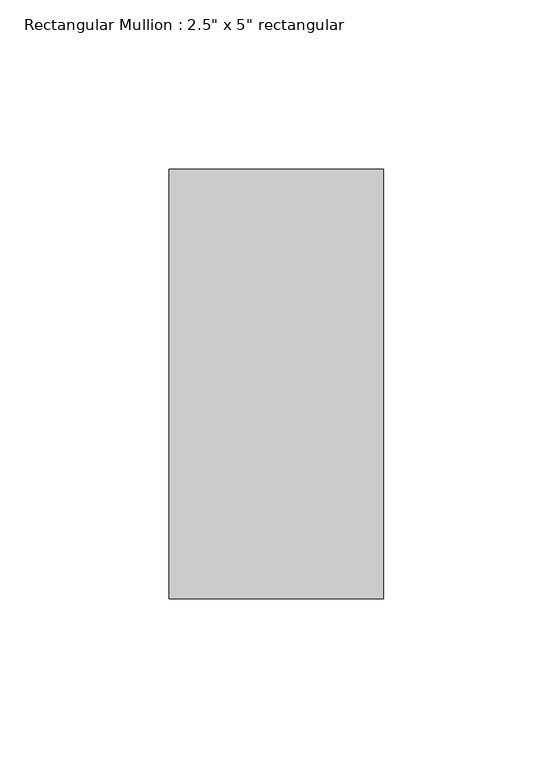
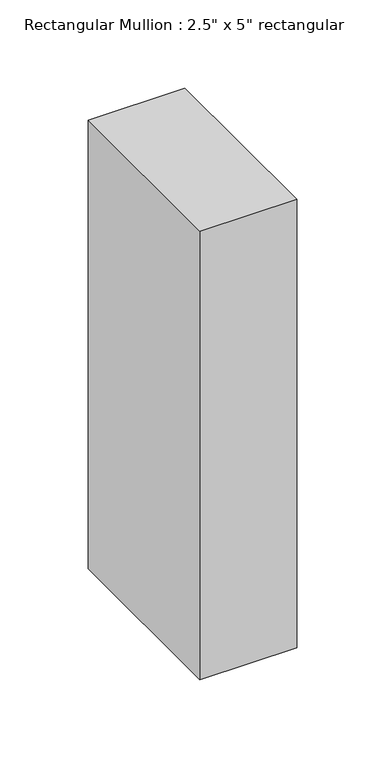
"""IFC4 building model written with IfcOpenShell, lengths in millimetres: member geometry."""

from ifc_helpers import new_model, si_unit, frame, origin, place, context, project, spatial, polyline, outline, extrude, source, transform, mapped, element, save


def member_9850ab14(model_context):
    return source(origin(), model_context, "Body", "SweptSolid", [
        extrude(outline(polyline([(31.75, 63.5), (31.75, -63.5), (-31.75, -63.5), (-31.75, 63.5), (31.75, 63.5)])), frame((0.0, 0.0, -311.15), z_axis=(0.0, 0.0, 1.0), x_axis=(1.0, 0.0, 0.0)), (0.0, 0.0, 1.0), 311.15),
    ])


if __name__ == "__main__":
    model = new_model("IFC4")
    model_context = context("Model", 3, world=origin())
    ifc_project = project(units=[si_unit("LENGTHUNIT", "METRE", prefix="MILLI")], contexts=[model_context])
    site = spatial("IfcSite", under=ifc_project)
    building = spatial("IfcBuilding", under=site)
    placement = place(None, origin())
    member_shape = member_9850ab14(model_context)
    element("IfcMember", 1, ObjectType="Rectangular Mullion : 2.5\" x 5\" rectangular", at=placement, inside=building, context=model_context, shape_type="MappedRepresentation", body=[
        mapped(member_shape, transform((0.0, 0.0, 0.0), x_axis=(1.0, 0.0, 0.0), y_axis=(0.0, 1.0, 0.0), z_axis=(0.0, 0.0, 1.0))),
    ])
    save(model, "model.ifc")

# Revit data of these elements
# Type "Rectangular Mullion : 2.5\" x 5\" rectangular"
#   built-in parameter 1007304 = 0.416667 (stored number, unit not read)
#   built-in parameter 1007301 = 0.104167 (stored number, unit not read)
#   built-in parameter 1007300 = 0.104167 (stored number, unit not read)
# Element 1 (IfcMember, "Rectangular Mullion : 2.5\" x 5\" rectangular")
#   Materials on its faces: "Aluminum"
# Materials
#   "Aluminum": class "Metal", colour RGB 247 247 247, transparency 0, Description = "Aluminum 6061", Cost = 0
